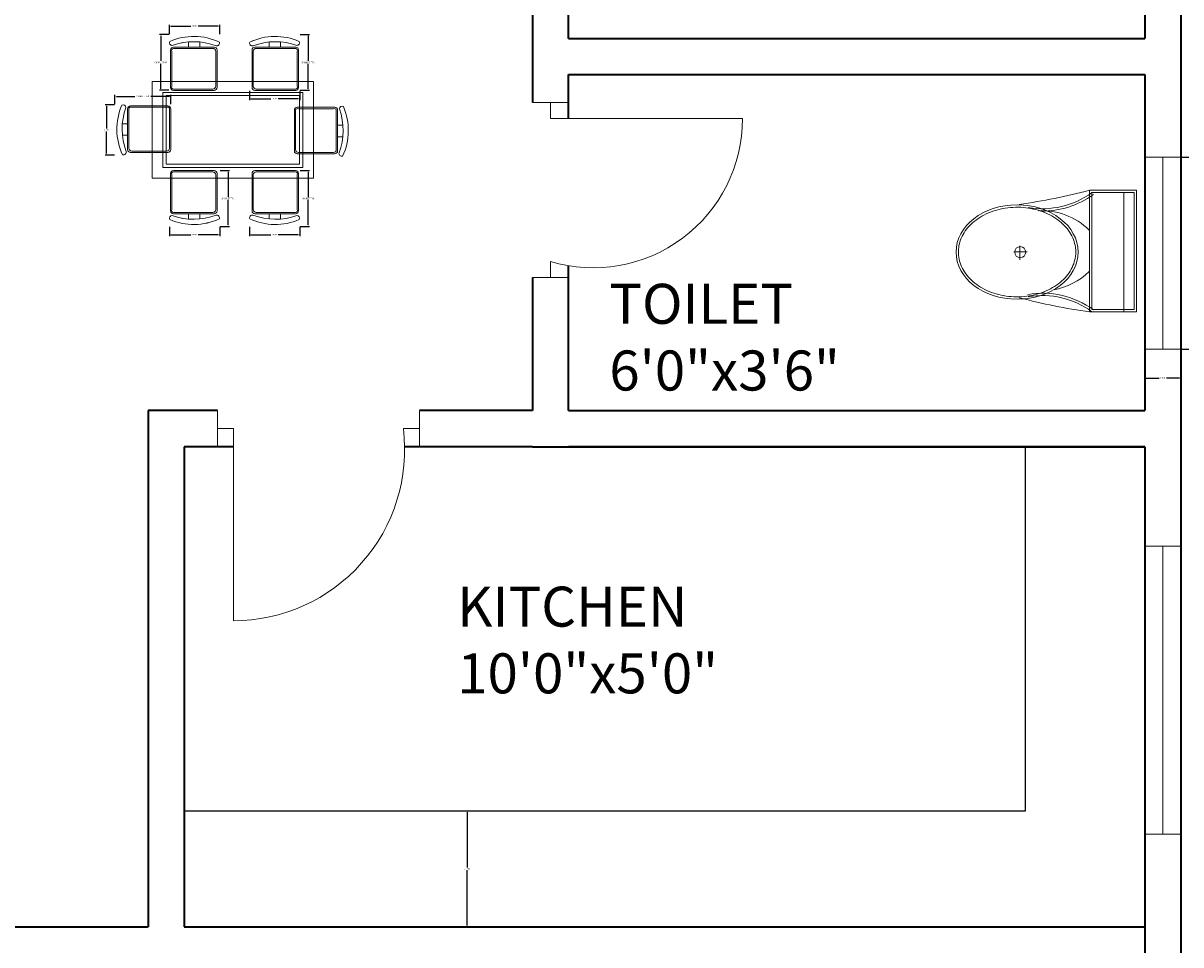
# Model space of a CAD drawing. Units: inches. Extents: x 2234 to 3001, y 1541 to 2386.
# Tile 10 of 12: x 2744 to 2888, y 2002 to 2118. Entities that reach past the tile are written whole.
import ezdxf

# ---------------------------------------------------------------- set-up
doc = ezdxf.new("R2010")
doc.units = ezdxf.units.IN
for name, color, linetype, lineweight in [('A-ANNO-DIMS', 2, 'Continuous', 18), ('A-AREA-IDEN', 7, 'Continuous', 18), ('A-DOOR', 3, 'Continuous', 18), ('A-FLOR-CASE', 8, 'Continuous', 25), ('A-FLOR-FIXT', 9, 'Continuous', 18), ('A-FURN', 9, 'Continuous', 13), ('A-GLAZ', 4, 'Continuous', 18), ('A-WALL', 7, 'Continuous', 35)]:
    doc.layers.add(name, color=color, linetype=linetype, lineweight=lineweight)
doc.styles.get("Standard").update_dxf_attribs({"font": 'arial.ttf'})
doc.dimstyles.get("Standard").update_dxf_attribs({"dimtxt": 0.18, "dimasz": 0.18, "dimexe": 0.18, "dimexo": 0.0625, "dimgap": 0.09, "dimtad": 0, "dimtih": 1, "dimtoh": 1, "dimdec": 4, "dimzin": 0, "dimdsep": 46, "dimtxsty": 'Standard', "dimcen": 0.09, "dimadec": 0, "dimazin": 0, "dimtfac": 1, "dimtdec": 4, "dimtofl": 0, "dimtmove": 0, "dimatfit": 3, "dimfxl": 1, "dimtolj": 1, "dimtzin": 0, "dimarcsym": 0})

# ---------------------------------------------------------------- blocks, each defined once
blk = doc.blocks.new('A$C31115884')
for p, q in [((283.1, 497.7), (223.4, 497.7)), ((257.5, 466.4), (257.5, 523.2)), ((0, 200), (0, 0)), ((520, 200), (0, 200)), ((520, 0), (520, 200)), ((10, 190), (10, 10)), ((510, 190), (10, 190)), ((510, 10), (510, 190)), ((510, 54.5), (0, 54.5)), ((10, 10), (510, 10)), ((0, 0), (520, 0))]:
    blk.add_line(p, q)
blk.add_circle((255.6, 496.4), 23.6)
for centre, radius, start, end in [((2777.7, -204.6), 2807, 165.4549, 171.7133), ((3237, 905), 2807, 188.2867, 194.5451), ((-294.5, 403.3), 364.7, 324.2091, 9.3499), ((-294.5, 403.3), 374.7, 324.2091, 9.3499), ((805.8, 403.3), 364.7, 170.6501, 215.7909), ((139.5, 406.2), 293.5, 315.8436, 2.6563), ((805.8, 403.3), 374.7, 179.2036, 215.7909), ((383.6, 406.2), 293.5, 190.2774, 224.1564)]:
    blk.add_arc(centre, radius, start, end)
blk.add_ellipse((256.2, 509.9), major_axis=(0, -260.7), ratio=0.772727)
blk.add_open_spline([(256.2, 259.2), (263.1, 259.2), (270, 259.7), (287.8, 262.3), (298.7, 265.1), (319.9, 273.1), (330.2, 278.4), (350.1, 291.1), (359.7, 298.7), (377.7, 315.9), (386.2, 325.5), (401.7, 346.6), (408.8, 358.1), (421.3, 382.5), (426.8, 395.5), (435.9, 422.4), (439.5, 436.4), (444.8, 465.1), (446.5, 479.7), (447.9, 509.2), (447.6, 524), (445, 553.3), (442.7, 567.8), (436.3, 596), (432.1, 609.7), (421.9, 636), (416, 648.6), (402.5, 672.1), (395, 683), (378.6, 703), (369.8, 712.1), (351.1, 728), (341.3, 734.8), (320.9, 746.2), (310.4, 750.7), (288.9, 757.3), (278, 759.4), (256, 761), (245, 760.6), (223.1, 757.2), (212.3, 754.3), (191.1, 746.1), (180.8, 740.7), (160.9, 727.8), (151.4, 720.1), (133.5, 702.7), (125.1, 693), (109.6, 671.7), (102.6, 660.2), (90.2, 635.7), (84.9, 622.7), (76, 595.6), (72.4, 581.6), (67.2, 552.9), (65.6, 538.2), (64.4, 508.8), (64.8, 494), (67.5, 464.7), (69.9, 450.2), (76.6, 422), (80.8, 408.3), (91.1, 382.2), (97.2, 369.7), (110.8, 346.3), (118.4, 335.4), (134.8, 315.6), (143.7, 306.7), (162.4, 290.9), (172.3, 284.2), (192.8, 273), (203.3, 268.6), (224.8, 262.2), (235.8, 260.2), (249.9, 259.3), (253, 259.2), (256.2, 259.2)], degree=3, knots=[0, 0, 0, 0, 0.110105, 0.110105, 0.285049, 0.285049, 0.459994, 0.459994, 0.634938, 0.634938, 0.809882, 0.809882, 0.984827, 0.984827, 1.159771, 1.159771, 1.334715, 1.334715, 1.50966, 1.50966, 1.684604, 1.684604, 1.859549, 1.859549, 2.034493, 2.034493, 2.209437, 2.209437, 2.384382, 2.384382, 2.559326, 2.559326, 2.73427, 2.73427, 2.909215, 2.909215, 3.084159, 3.084159, 3.259103, 3.259103, 3.434048, 3.434048, 3.608992, 3.608992, 3.783936, 3.783936, 3.958881, 3.958881, 4.133825, 4.133825, 4.30877, 4.30877, 4.483714, 4.483714, 4.658658, 4.658658, 4.833603, 4.833603, 5.008547, 5.008547, 5.183491, 5.183491, 5.358436, 5.358436, 5.53338, 5.53338, 5.708324, 5.708324, 5.883269, 5.883269, 6.058213, 6.058213, 6.233158, 6.233158, 6.283185, 6.283185, 6.283185, 6.283185])
blk = doc.blocks.new('TABLE-DINING-RECT')
for points in [[(0, 12.09), (20.14, 12.09), (20.14, 0), (0, 0)], [(0, 12.09), (20.14, 12.09), (20.14, 0), (0, 0)], [(1.34, 10.74), (18.8, 10.74), (18.8, 1.34), (1.34, 1.34)], [(1.34, 10.74), (18.8, 10.74), (18.8, 1.34), (1.34, 1.34)], [(1.75, 10.34), (18.4, 10.34), (18.4, 1.75), (1.75, 1.75)], [(1.75, 10.34), (18.4, 10.34), (18.4, 1.75), (1.75, 1.75)]]:
    blk.add_lwpolyline(points, close=True)
blk = doc.blocks.new('CHAIR-DINING-A')
for points in [[(5.76, 1.34, 0.414214), (6.12, 1.7), (6.12, 6.38, 0.414214), (5.76, 6.74), (0.67, 6.74, 0.414214), (0.31, 6.38), (0.31, 1.7, 0.414214), (0.67, 1.34), (5.76, 1.34)], [(5.76, 1.34, 0.414214), (6.12, 1.7), (6.12, 6.38, 0.414214), (5.76, 6.74), (0.67, 6.74, 0.414214), (0.31, 6.38), (0.31, 1.7, 0.414214), (0.67, 1.34), (5.76, 1.34)], [(5.92, 1.12, -0.175809), (0.43, 1.16, 0.578392), (0.02, 0.71, 0.214524), (6.21, 0.62, 0.552014), (5.92, 1.12, -0.065079)], [(5.92, 1.12, -0.175809), (0.43, 1.16, 0.578392), (0.02, 0.71, 0.214524), (6.21, 0.62, 0.552014), (5.92, 1.12, -0.065079)], [(2.45, 1.34), (2.45, 0.7, -0.064759)], [(2.45, 1.34), (2.45, 0.7, -0.064759)]]:
    blk.add_lwpolyline(points, format="xyb")
blk.add_lwpolyline([(5.76, 1.5), (0.83, 1.5, -0.414214), (0.47, 1.86), (0.47, 6.22, -0.414214), (0.83, 6.58), (5.76, 6.58, -0.512069), (5.95, 6.22), (5.95, 1.86, -0.512069)], format="xyb", close=True)
blk.add_lwpolyline([(5.76, 1.5), (0.83, 1.5, -0.414214), (0.47, 1.86), (0.47, 6.22, -0.414214), (0.83, 6.58), (5.76, 6.58, -0.512069), (5.95, 6.22), (5.95, 1.86, -0.512069)], format="xyb", close=True)
blk.add_lwpolyline([(3.88, 0.69), (3.88, 1.34)])
blk.add_lwpolyline([(3.88, 0.69), (3.88, 1.34)])
blk = doc.blocks.new('CHAIR-DINING-C')
for points in [[(1.16, 0.43, -0.578392), (0.71, 0.02, -0.214524), (0.62, 6.21, -0.552014), (1.12, 5.92, 0.175809), (1.16, 0.43)], [(1.34, 5.76, -0.414214), (1.7, 6.11), (6.38, 6.11, -0.414214), (6.74, 5.76), (6.74, 0.66, -0.414214), (6.38, 0.31), (1.7, 0.31, -0.414214), (1.34, 0.66), (1.34, 5.76)], [(1.34, 2.45), (0.7, 2.45, 0.064759)]]:
    blk.add_lwpolyline(points, format="xyb")
blk.add_lwpolyline([(1.5, 5.76), (1.5, 0.83, 0.414214), (1.86, 0.47), (6.22, 0.47, 0.414214), (6.58, 0.83), (6.58, 5.76, 0.512069), (6.22, 5.95), (1.86, 5.95, 0.512069)], format="xyb", close=True)
blk.add_lwpolyline([(0.69, 3.88), (1.34, 3.88)])
blk = doc.blocks.new('CHAIR-DINING-D')
for points in [[(0.43, 5.57, -0.578392), (0.02, 6.03, -0.214524), (6.21, 6.11, -0.552014), (5.92, 5.62, 0.175809), (0.43, 5.57)], [(2.45, 5.4), (2.45, 6.04, 0.064759)], [(5.76, 5.4, -0.414214), (6.12, 5.04), (6.12, 0.36, -0.414214), (5.76, 0), (0.67, 0, -0.414214), (0.31, 0.36), (0.31, 5.04, -0.414214), (0.67, 5.4), (5.76, 5.4)]]:
    blk.add_lwpolyline(points, format="xyb")
blk.add_lwpolyline([(3.88, 6.05), (3.88, 5.4)])
blk.add_lwpolyline([(5.76, 5.24), (0.83, 5.24, 0.414214), (0.47, 4.88), (0.47, 0.52, 0.414214), (0.83, 0.16), (5.76, 0.16, 0.512069), (5.95, 0.52), (5.95, 4.88, 0.512069)], format="xyb", close=True)
blk = doc.blocks.new('CHAIR-DINING-E')
for points in [[(5.76, 1.34, 0.414214), (6.12, 1.7), (6.12, 6.38, 0.414214), (5.76, 6.74), (0.67, 6.74, 0.414214), (0.31, 6.38), (0.31, 1.7, 0.414214), (0.67, 1.34), (5.76, 1.34)], [(5.92, 1.12, -0.175809), (0.43, 1.16, 0.578392), (0.02, 0.71, 0.214524), (6.21, 0.62, 0.552014), (5.92, 1.12, -0.065079)], [(2.45, 1.34), (2.45, 0.7, -0.064759)]]:
    blk.add_lwpolyline(points, format="xyb")
blk.add_lwpolyline([(5.76, 1.5), (0.83, 1.5, -0.414214), (0.47, 1.86), (0.47, 6.22, -0.414214), (0.83, 6.58), (5.76, 6.58, -0.512069), (5.95, 6.22), (5.95, 1.86, -0.512069)], format="xyb", close=True)
blk.add_lwpolyline([(3.88, 0.69), (3.88, 1.34)])
blk = doc.blocks.new('CHAIR-DINING-G')
for points in [[(5.58, 1.34), (0.49, 1.34, -0.414214), (0.13, 1.7), (0.13, 6.38, -0.414214), (0.49, 6.74), (5.58, 6.74, -0.414214), (5.94, 6.38), (5.94, 1.7, -0.414214), (5.58, 1.34)], [(5.82, 1.16, -0.578392), (6.23, 0.71, -0.214524), (0.04, 0.62, -0.552014), (0.33, 1.12, 0.175809), (5.82, 1.16)], [(3.79, 1.34), (3.79, 0.7, 0.064759)]]:
    blk.add_lwpolyline(points, format="xyb")
blk.add_lwpolyline([(0.49, 1.5), (5.42, 1.5, 0.414214), (5.78, 1.86), (5.78, 6.22, 0.414214), (5.42, 6.58), (0.49, 6.58, 0.512069), (0.29, 6.22), (0.29, 1.86, 0.512069)], format="xyb", close=True)
blk.add_lwpolyline([(2.37, 0.69), (2.37, 1.34)])
blk = doc.blocks.new('CHAIR-DINING-H')
for points in [[(1.16, 0.43, -0.578392), (0.71, 0.02, -0.214524), (0.62, 6.21, -0.552014), (1.12, 5.92, 0.175809), (1.16, 0.43)], [(1.34, 5.76, -0.414214), (1.7, 6.11), (6.38, 6.11, -0.414214), (6.74, 5.76), (6.74, 0.66, -0.414214), (6.38, 0.31), (1.7, 0.31, -0.414214), (1.34, 0.66), (1.34, 5.76)], [(1.34, 2.45), (0.7, 2.45, 0.064759)]]:
    blk.add_lwpolyline(points, format="xyb")
blk.add_lwpolyline([(1.5, 5.76), (1.5, 0.83, 0.414214), (1.86, 0.47), (6.22, 0.47, 0.414214), (6.58, 0.83), (6.58, 5.76, 0.512069), (6.22, 5.95), (1.86, 5.95, 0.512069)], format="xyb", close=True)
blk.add_lwpolyline([(0.69, 3.88), (1.34, 3.88)])
blk = doc.blocks.new('CHAIR-DINING-I')
for points in [[(0.33, 5.62, -0.175809), (5.82, 5.57, 0.578392), (6.23, 6.03, 0.214524), (0.04, 6.11, 0.552014), (0.33, 5.62, -0.065079)], [(3.79, 5.4), (3.79, 6.04, -0.064759)], [(5.58, 5.4), (0.49, 5.4, 0.414214), (0.13, 5.04), (0.13, 0.36, 0.414214), (0.49, 0), (5.58, 0, 0.414214), (5.94, 0.36), (5.94, 5.04, 0.414214), (5.58, 5.4)]]:
    blk.add_lwpolyline(points, format="xyb")
blk.add_lwpolyline([(2.37, 6.05), (2.37, 5.4)])
blk.add_lwpolyline([(0.49, 5.24), (5.42, 5.24, -0.414214), (5.78, 4.88), (5.78, 0.52, -0.414214), (5.42, 0.16), (0.49, 0.16, -0.512069), (0.29, 0.52), (0.29, 4.88, -0.512069)], format="xyb", close=True)
blk = doc.blocks.new('WIN-24-A')
for p, q in [((0, 24), (4.5, 24)), ((4.5, 24), (2.25, 24)), ((2.25, 24), (2.25, 0)), ((2.25, 0), (0, 0)), ((0, 0), (4.5, 0))]:
    blk.add_line(p, q)
blk = doc.blocks.new('WIN-36')
for p, q in [((0, 36), (4.5, 36)), ((4.5, 36), (2.25, 36)), ((2.25, 36), (2.25, 0)), ((2.25, 0), (0, 0)), ((0, 0), (4.5, 0))]:
    blk.add_line(p, q)
blk = doc.blocks.new('*D29')
at = {"layer": 'A-ANNO-DIMS', "color": 0, "lineweight": -2, "transparency": 16777216}
for p, q in [((2888.32, 2100.78), (2892.03, 2100.78)), ((2891.85, 2100.6), (2891.85, 2088.96)), ((2891.85, 2076.96), (2891.85, 2088.6)), ((2888.32, 2076.78), (2892.03, 2076.78))]:
    blk.add_line(p, q, dxfattribs=at)
at = {"layer": 'A-ANNO-DIMS', "color": 0, "transparency": 16777216}
for points in [[(2891.82, 2100.6), (2891.88, 2100.6), (2891.85, 2100.78)], [(2891.82, 2076.96), (2891.88, 2076.96), (2891.85, 2076.78)]]:
    blk.add_solid(points, dxfattribs=at)
at = {"layer": 'Defpoints', "color": 0, "transparency": 16777216}
for p in [(2888.25, 2100.78), (2888.25, 2076.78), (2891.85, 2076.78)]:
    blk.add_point(p, dxfattribs=at)
at = {"layer": 'A-ANNO-DIMS', "color": 0, "transparency": 16777216, "insert": (2891.85, 2088.78), "char_height": 0.18, "attachment_point": 5}
blk.add_mtext('\\A1;W-A 24 TYP.', dxfattribs=at)
blk = doc.blocks.new('*D30')
at = {"layer": 'A-ANNO-DIMS', "color": 0, "lineweight": -2, "transparency": 16777216}
for p, q in [((2883.75, 2076.72), (2883.75, 2073)), ((2888.25, 2076.72), (2888.25, 2073)), ((2883.93, 2073.18), (2885.55, 2073.18)), ((2888.07, 2073.18), (2886.46, 2073.18))]:
    blk.add_line(p, q, dxfattribs=at)
at = {"layer": 'A-ANNO-DIMS', "color": 0, "transparency": 16777216}
for points in [[(2883.93, 2073.21), (2883.93, 2073.15), (2883.75, 2073.18)], [(2888.07, 2073.21), (2888.07, 2073.15), (2888.25, 2073.18)]]:
    blk.add_solid(points, dxfattribs=at)
at = {"layer": 'Defpoints', "color": 0, "transparency": 16777216}
for p in [(2883.75, 2076.78), (2888.25, 2076.78), (2883.75, 2073.18)]:
    blk.add_point(p, dxfattribs=at)
at = {"layer": 'A-ANNO-DIMS', "color": 0, "transparency": 16777216, "insert": (2886, 2073.18), "char_height": 0.18, "attachment_point": 5}
blk.add_mtext('\\A1;5 TYP.', dxfattribs=at)
blk = doc.blocks.new('*D47')
at = {"layer": 'A-ANNO-DIMS', "color": 0, "lineweight": -2, "transparency": 16777216}
for p, q in [((2778.25, 2116.11), (2779.41, 2116.11)), ((2779.23, 2115.93), (2779.23, 2112.81)), ((2779.23, 2109.32), (2779.23, 2112.44)), ((2778.25, 2109.14), (2779.41, 2109.14))]:
    blk.add_line(p, q, dxfattribs=at)
at = {"layer": 'A-ANNO-DIMS', "color": 0, "transparency": 16777216}
for points in [[(2779.2, 2115.93), (2779.26, 2115.93), (2779.23, 2116.11)], [(2779.2, 2109.32), (2779.26, 2109.32), (2779.23, 2109.14)]]:
    blk.add_solid(points, dxfattribs=at)
at = {"layer": 'Defpoints', "color": 0, "transparency": 16777216}
for p in [(2778.18, 2116.11), (2779.23, 2116.11), (2778.18, 2109.14)]:
    blk.add_point(p, dxfattribs=at)
at = {"layer": 'A-ANNO-DIMS', "color": 0, "transparency": 16777216, "insert": (2779.23, 2112.62), "char_height": 0.18, "attachment_point": 5}
blk.add_mtext('\\A1;CHAIR D 7 TYP.', dxfattribs=at)
blk = doc.blocks.new('*D48')
at = {"layer": 'A-ANNO-DIMS', "color": 0, "lineweight": -2, "transparency": 16777216}
for p, q in [((2771.9, 2109.07), (2771.9, 2107.91)), ((2778.18, 2109.07), (2778.18, 2107.91)), ((2772.08, 2108.09), (2774.58, 2108.09)), ((2778, 2108.09), (2775.5, 2108.09))]:
    blk.add_line(p, q, dxfattribs=at)
at = {"layer": 'A-ANNO-DIMS', "color": 0, "transparency": 16777216}
for points in [[(2772.08, 2108.12), (2772.08, 2108.06), (2771.9, 2108.09)], [(2778, 2108.12), (2778, 2108.06), (2778.18, 2108.09)]]:
    blk.add_solid(points, dxfattribs=at)
at = {"layer": 'Defpoints', "color": 0, "transparency": 16777216}
for p in [(2771.9, 2109.14), (2778.18, 2109.14), (2778.18, 2108.09)]:
    blk.add_point(p, dxfattribs=at)
at = {"layer": 'A-ANNO-DIMS', "color": 0, "transparency": 16777216, "insert": (2775.04, 2108.09), "char_height": 0.18, "attachment_point": 5}
blk.add_mtext('\\A1;6 TYP.', dxfattribs=at)
blk = doc.blocks.new('*D49')
at = {"layer": 'A-ANNO-DIMS', "color": 0, "lineweight": -2, "transparency": 16777216}
for p, q in [((2778.25, 2099.11), (2779.41, 2099.11)), ((2779.23, 2098.93), (2779.23, 2095.8)), ((2779.23, 2092.31), (2779.23, 2095.44)), ((2778.25, 2092.13), (2779.41, 2092.13))]:
    blk.add_line(p, q, dxfattribs=at)
at = {"layer": 'A-ANNO-DIMS', "color": 0, "transparency": 16777216}
for points in [[(2779.2, 2098.93), (2779.26, 2098.93), (2779.23, 2099.11)], [(2779.2, 2092.31), (2779.26, 2092.31), (2779.23, 2092.13)]]:
    blk.add_solid(points, dxfattribs=at)
at = {"layer": 'Defpoints', "color": 0, "transparency": 16777216}
for p in [(2778.18, 2099.11), (2779.23, 2099.11), (2778.18, 2092.13)]:
    blk.add_point(p, dxfattribs=at)
at = {"layer": 'A-ANNO-DIMS', "color": 0, "transparency": 16777216, "insert": (2779.23, 2095.62), "char_height": 0.18, "attachment_point": 5}
blk.add_mtext('\\A1;CHAIR E 7 TYP.', dxfattribs=at)
blk = doc.blocks.new('*D50')
at = {"layer": 'A-ANNO-DIMS', "color": 0, "lineweight": -2, "transparency": 16777216}
for p, q in [((2771.9, 2092.07), (2771.9, 2090.91)), ((2778.18, 2092.07), (2778.18, 2090.91)), ((2772.08, 2091.09), (2774.58, 2091.09)), ((2778, 2091.09), (2775.5, 2091.09))]:
    blk.add_line(p, q, dxfattribs=at)
at = {"layer": 'A-ANNO-DIMS', "color": 0, "transparency": 16777216}
for points in [[(2772.08, 2091.12), (2772.08, 2091.06), (2771.9, 2091.09)], [(2778, 2091.12), (2778, 2091.06), (2778.18, 2091.09)]]:
    blk.add_solid(points, dxfattribs=at)
at = {"layer": 'Defpoints', "color": 0, "transparency": 16777216}
for p in [(2771.9, 2092.13), (2778.18, 2092.13), (2778.18, 2091.09)]:
    blk.add_point(p, dxfattribs=at)
at = {"layer": 'A-ANNO-DIMS', "color": 0, "transparency": 16777216, "insert": (2775.04, 2091.09), "char_height": 0.18, "attachment_point": 5}
blk.add_mtext('\\A1;6 TYP.', dxfattribs=at)
blk = doc.blocks.new('*D53')
at = {"layer": 'A-ANNO-DIMS', "color": 0, "lineweight": -2, "transparency": 16777216}
for p, q in [((2768.25, 2099.11), (2769.41, 2099.11)), ((2769.23, 2098.93), (2769.23, 2095.8)), ((2769.23, 2092.31), (2769.23, 2095.44)), ((2768.25, 2092.13), (2769.41, 2092.13))]:
    blk.add_line(p, q, dxfattribs=at)
at = {"layer": 'A-ANNO-DIMS', "color": 0, "transparency": 16777216}
for points in [[(2769.2, 2098.93), (2769.26, 2098.93), (2769.23, 2099.11)], [(2769.2, 2092.31), (2769.26, 2092.31), (2769.23, 2092.13)]]:
    blk.add_solid(points, dxfattribs=at)
at = {"layer": 'Defpoints', "color": 0, "transparency": 16777216}
for p in [(2768.19, 2099.11), (2769.23, 2099.11), (2768.19, 2092.13)]:
    blk.add_point(p, dxfattribs=at)
at = {"layer": 'A-ANNO-DIMS', "color": 0, "transparency": 16777216, "insert": (2769.23, 2095.62), "char_height": 0.18, "attachment_point": 5}
blk.add_mtext('\\A1;CHAIR G 7 TYP.', dxfattribs=at)
blk = doc.blocks.new('*D54')
at = {"layer": 'A-ANNO-DIMS', "color": 0, "lineweight": -2, "transparency": 16777216}
for p, q in [((2761.9, 2092.07), (2761.9, 2090.91)), ((2768.19, 2092.07), (2768.19, 2090.91)), ((2762.08, 2091.09), (2764.59, 2091.09)), ((2768.01, 2091.09), (2765.5, 2091.09))]:
    blk.add_line(p, q, dxfattribs=at)
at = {"layer": 'A-ANNO-DIMS', "color": 0, "transparency": 16777216}
for points in [[(2762.08, 2091.12), (2762.08, 2091.06), (2761.9, 2091.09)], [(2768.01, 2091.12), (2768.01, 2091.06), (2768.19, 2091.09)]]:
    blk.add_solid(points, dxfattribs=at)
at = {"layer": 'Defpoints', "color": 0, "transparency": 16777216}
for p in [(2761.9, 2092.13), (2768.19, 2092.13), (2768.19, 2091.09)]:
    blk.add_point(p, dxfattribs=at)
at = {"layer": 'A-ANNO-DIMS', "color": 0, "transparency": 16777216, "insert": (2765.04, 2091.09), "char_height": 0.18, "attachment_point": 5}
blk.add_mtext('\\A1;6 TYP.', dxfattribs=at)
blk = doc.blocks.new('*D55')
at = {"layer": 'A-ANNO-DIMS', "color": 0, "lineweight": -2, "transparency": 16777216}
for p, q in [((2755.11, 2107.4), (2755.11, 2108.56)), ((2762.08, 2107.4), (2762.08, 2108.56)), ((2755.29, 2108.38), (2757.58, 2108.38)), ((2761.9, 2108.38), (2759.6, 2108.38))]:
    blk.add_line(p, q, dxfattribs=at)
at = {"layer": 'A-ANNO-DIMS', "color": 0, "transparency": 16777216}
for points in [[(2755.29, 2108.41), (2755.29, 2108.35), (2755.11, 2108.38)], [(2761.9, 2108.41), (2761.9, 2108.35), (2762.08, 2108.38)]]:
    blk.add_solid(points, dxfattribs=at)
at = {"layer": 'Defpoints', "color": 0, "transparency": 16777216}
for p in [(2755.11, 2107.33), (2762.08, 2108.38), (2762.08, 2107.33)]:
    blk.add_point(p, dxfattribs=at)
at = {"layer": 'A-ANNO-DIMS', "color": 0, "transparency": 16777216, "insert": (2758.59, 2108.38), "char_height": 0.18, "attachment_point": 5}
blk.add_mtext('\\A1;CHAIR H 7 TYP.', dxfattribs=at)
blk = doc.blocks.new('*D56')
at = {"layer": 'A-ANNO-DIMS', "color": 0, "lineweight": -2, "transparency": 16777216}
for p, q in [((2755.04, 2107.33), (2753.88, 2107.33)), ((2754.06, 2107.15), (2754.06, 2104.37)), ((2754.06, 2101.23), (2754.06, 2104.01)), ((2755.04, 2101.05), (2753.88, 2101.05))]:
    blk.add_line(p, q, dxfattribs=at)
at = {"layer": 'A-ANNO-DIMS', "color": 0, "transparency": 16777216}
for points in [[(2754.03, 2107.15), (2754.09, 2107.15), (2754.06, 2107.33)], [(2754.03, 2101.23), (2754.09, 2101.23), (2754.06, 2101.05)]]:
    blk.add_solid(points, dxfattribs=at)
at = {"layer": 'Defpoints', "color": 0, "transparency": 16777216}
for p in [(2754.06, 2107.33), (2755.11, 2107.33), (2755.11, 2101.05)]:
    blk.add_point(p, dxfattribs=at)
at = {"layer": 'A-ANNO-DIMS', "color": 0, "transparency": 16777216, "insert": (2754.06, 2104.19), "char_height": 0.18, "attachment_point": 5}
blk.add_mtext('\\A1;6 TYP.', dxfattribs=at)
blk = doc.blocks.new('*D57')
at = {"layer": 'A-ANNO-DIMS', "color": 0, "lineweight": -2, "transparency": 16777216}
for p, q in [((2761.84, 2116.11), (2760.67, 2116.11)), ((2760.85, 2115.93), (2760.85, 2112.81)), ((2760.85, 2109.32), (2760.85, 2112.44)), ((2761.84, 2109.14), (2760.67, 2109.14))]:
    blk.add_line(p, q, dxfattribs=at)
at = {"layer": 'A-ANNO-DIMS', "color": 0, "transparency": 16777216}
for points in [[(2760.82, 2115.93), (2760.88, 2115.93), (2760.85, 2116.11)], [(2760.82, 2109.32), (2760.88, 2109.32), (2760.85, 2109.14)]]:
    blk.add_solid(points, dxfattribs=at)
at = {"layer": 'Defpoints', "color": 0, "transparency": 16777216}
for p in [(2760.85, 2116.11), (2761.9, 2116.11), (2761.9, 2109.14)]:
    blk.add_point(p, dxfattribs=at)
at = {"layer": 'A-ANNO-DIMS', "color": 0, "transparency": 16777216, "insert": (2760.85, 2112.62), "char_height": 0.18, "attachment_point": 5}
blk.add_mtext('\\A1;CHAIR I 7 TYP.', dxfattribs=at)
blk = doc.blocks.new('*D58')
at = {"layer": 'A-ANNO-DIMS', "color": 0, "lineweight": -2, "transparency": 16777216}
for p, q in [((2761.9, 2116.17), (2761.9, 2117.34)), ((2768.19, 2116.17), (2768.19, 2117.34)), ((2762.08, 2117.16), (2764.59, 2117.16)), ((2768.01, 2117.16), (2765.5, 2117.16))]:
    blk.add_line(p, q, dxfattribs=at)
at = {"layer": 'A-ANNO-DIMS', "color": 0, "transparency": 16777216}
for points in [[(2762.08, 2117.19), (2762.08, 2117.13), (2761.9, 2117.16)], [(2768.01, 2117.19), (2768.01, 2117.13), (2768.19, 2117.16)]]:
    blk.add_solid(points, dxfattribs=at)
at = {"layer": 'Defpoints', "color": 0, "transparency": 16777216}
for p in [(2761.9, 2116.11), (2768.19, 2117.16), (2768.19, 2116.11)]:
    blk.add_point(p, dxfattribs=at)
at = {"layer": 'A-ANNO-DIMS', "color": 0, "transparency": 16777216, "insert": (2765.04, 2117.16), "char_height": 0.18, "attachment_point": 5}
blk.add_mtext('\\A1;6 TYP.', dxfattribs=at)
blk = doc.blocks.new('*D73')
at = {"layer": 'A-ANNO-DIMS', "color": 0, "lineweight": -2, "transparency": 16777216}
for p, q in [((2763.82, 2019.11), (2799.28, 2019.11)), ((2799.1, 2018.93), (2799.1, 2012.04)), ((2799.1, 2004.79), (2799.1, 2011.68)), ((2763.82, 2004.61), (2799.28, 2004.61))]:
    blk.add_line(p, q, dxfattribs=at)
at = {"layer": 'A-ANNO-DIMS', "color": 0, "transparency": 16777216}
for points in [[(2799.07, 2018.93), (2799.13, 2018.93), (2799.1, 2019.11)], [(2799.07, 2004.79), (2799.13, 2004.79), (2799.1, 2004.61)]]:
    blk.add_solid(points, dxfattribs=at)
at = {"layer": 'Defpoints', "color": 0, "transparency": 16777216}
for p in [(2763.75, 2019.11), (2763.75, 2004.61), (2799.1, 2004.61)]:
    blk.add_point(p, dxfattribs=at)
at = {"layer": 'A-ANNO-DIMS', "color": 0, "transparency": 16777216, "insert": (2799.1, 2011.86), "char_height": 0.18, "attachment_point": 5}
blk.add_mtext('\\A1;14.498', dxfattribs=at)

msp = doc.modelspace()

# ---------------------------------------------------------------- linework, layer by layer
at = {"layer": 'A-DOOR'}
for p, q in [((2811.7534, 2107.6086), (2807.2534, 2107.6086)), ((2807.2534, 2107.6086), (2809.5034, 2107.6086)), ((2809.5034, 2107.6086), (2809.5034, 2105.6086)), ((2809.5034, 2105.6086), (2833.5034, 2105.6086)), ((2809.5034, 2085.7488), (2809.5034, 2087.7488)), ((2811.7534, 2085.7488), (2807.2534, 2085.7488)), ((2807.2534, 2085.7488), (2809.5034, 2085.7488)), ((2767.8978, 2064.611), (2767.8978, 2069.111)), ((2767.8978, 2069.111), (2767.8978, 2066.861)), ((2793.1311, 2064.611), (2793.1311, 2069.111)), ((2793.1311, 2069.111), (2793.1311, 2066.861)), ((2767.8978, 2066.861), (2769.8978, 2066.861)), ((2769.8978, 2066.861), (2769.8978, 2042.861)), ((2793.1311, 2066.861), (2791.1311, 2066.861))]:
    msp.add_line(p, q, dxfattribs=at)
for centre, radius, start, end in [((2814.8582, 2105.6086), 18.6453, 253.310145, 0), ((2769.8978, 2064.2539), 21.3928, 270, 7.000088)]:
    msp.add_arc(centre, radius, start, end, dxfattribs=at)
at = {"layer": 'A-FLOR-CASE'}
for p, q in [((2868.8394, 2019.1088), (2868.8394, 2064.611)), ((2763.7534, 2019.1088), (2868.8394, 2019.1088))]:
    msp.add_line(p, q, dxfattribs=at)
at = {"layer": 'A-FURN'}
for points in [[(2762.2461, 2114.7519, -0.17580919), (2767.7328, 2114.7104, 0.57839206), (2768.1484, 2115.1674, 0.21452438), (2761.9552, 2115.2505, 0.55201397), (2762.2461, 2114.7519, -0.06507904)], [(2772.3518, 2114.7104, -0.57839206), (2771.9361, 2115.1674, -0.21452438), (2778.1294, 2115.2505, -0.55201397), (2777.8384, 2114.7519, 0.1758092), (2772.3518, 2114.7104)], [(2767.5, 2114.5317), (2762.4064, 2114.5317, 0.41421356), (2762.05, 2114.1754), (2762.05, 2109.4919, 0.41421356), (2762.4064, 2109.1355), (2767.5, 2109.1355, 0.41421356), (2767.8563, 2109.4919), (2767.8563, 2114.1754, 0.41421356), (2767.5, 2114.5317)], [(2765.7109, 2114.5317), (2765.7109, 2115.1759, -0.06475861)], [(2777.6782, 2114.5317, -0.41421356), (2778.0345, 2114.1754), (2778.0345, 2109.4919, -0.41421356), (2777.6782, 2109.1355), (2772.5846, 2109.1355, -0.41421356), (2772.2282, 2109.4919), (2772.2282, 2114.1754, -0.41421356), (2772.5846, 2114.5317), (2777.6782, 2114.5317)], [(2774.3737, 2114.5317), (2774.3737, 2115.1759, 0.06475861)], [(2767.5, 2093.7125), (2762.4064, 2093.7125, -0.41421356), (2762.05, 2094.0689), (2762.05, 2098.7524, -0.41421356), (2762.4064, 2099.1087), (2767.5, 2099.1087, -0.41421356), (2767.8563, 2098.7524), (2767.8563, 2094.0689, -0.41421356), (2767.5, 2093.7125)], [(2767.7328, 2093.5339, -0.57839206), (2768.1484, 2093.0768, -0.21452438), (2761.9552, 2092.9937, -0.55201397), (2762.2461, 2093.4923, 0.17580929), (2767.7328, 2093.5339)], [(2765.7109, 2093.7125), (2765.7109, 2093.0683, 0.06475861)]]:
    msp.add_lwpolyline(points, format="xyb", dxfattribs=at)
for points in [[(2762.4085, 2114.3712), (2767.3394, 2114.3712, -0.41421356), (2767.6958, 2114.0148), (2767.6958, 2109.6524, -0.41421356), (2767.3394, 2109.2961), (2762.4085, 2109.2961, -0.51206948), (2762.2106, 2109.6524), (2762.2106, 2114.0148, -0.51206948)], [(2777.676, 2114.3712), (2772.7451, 2114.3712, 0.41421356), (2772.3888, 2114.0148), (2772.3888, 2109.6524, 0.41421356), (2772.7451, 2109.2961), (2777.676, 2109.2961, 0.51206948), (2777.874, 2109.6524), (2777.874, 2114.0148, 0.51206948)], [(2762.4085, 2093.8731), (2767.3394, 2093.8731, 0.41421356), (2767.6958, 2094.2294), (2767.6958, 2098.5918, 0.41421356), (2767.3394, 2098.9482), (2762.4085, 2098.9482, 0.51206948), (2762.2106, 2098.5918), (2762.2106, 2094.2294, 0.51206948)]]:
    msp.add_lwpolyline(points, format="xyb", close=True, dxfattribs=at)
for points in [[(2764.2851, 2115.1876), (2764.2851, 2114.5317)], [(2775.7995, 2115.1876), (2775.7995, 2114.5317)], [(2764.2851, 2093.0566), (2764.2851, 2093.7125)]]:
    msp.add_lwpolyline(points, dxfattribs=at)
at = {"layer": 'A-WALL'}
for p, q in [((2888.2534, 2298.611), (2888.2534, 1702.111)), ((2807.2534, 2157.611), (2807.2534, 2107.6086)), ((2811.7534, 2115.611), (2811.7534, 2157.611)), ((2883.7534, 2157.611), (2883.7534, 2115.611)), ((2811.7534, 2115.611), (2883.7534, 2115.611)), ((2811.7534, 2111.111), (2883.7534, 2111.111)), ((2811.7534, 2105.6086), (2811.7534, 2111.111)), ((2883.7534, 2111.111), (2883.7534, 2069.111)), ((2811.7534, 2069.111), (2811.7534, 2087.2236)), ((2807.2534, 2085.7488), (2807.2534, 2069.111)), ((2759.2534, 2069.111), (2759.2534, 2064.611)), ((2767.8978, 2069.111), (2759.2534, 2069.111)), ((2807.2534, 2069.111), (2793.1311, 2069.111)), ((2811.7534, 2069.111), (2883.7534, 2069.111)), ((2759.2534, 2064.611), (2759.2534, 2004.611)), ((2763.7534, 2064.611), (2763.7534, 2004.611)), ((2769.8978, 2064.611), (2763.7534, 2064.611)), ((2807.2534, 2064.611), (2791.2876, 2064.611)), ((2807.2534, 2064.611), (2883.7534, 2064.611)), ((2883.7534, 2064.611), (2811.7534, 2064.611)), ((2883.7534, 2064.611), (2883.7534, 1940.111)), ((2636.7879, 2004.611), (2759.2534, 2004.611)), ((2763.7534, 2004.611), (2883.7534, 2004.611))]:
    msp.add_line(p, q, dxfattribs=at)

# ---------------------------------------------------------------- block references
at = {"layer": 'A-FLOR-FIXT', "xscale": 0.0292470664339069, "yscale": 0.0292470664339069, "zscale": 0.0292470664339069, "rotation": 89.99999999999999}
msp.add_blockref('A$C31115884', (2882.7092, 2081.4404), dxfattribs=at)
at = {"layer": 'A-FURN'}
for name, p in [('CHAIR-DINING-I', (2761.9165, 2109.1359)), ('CHAIR-DINING-D', (2771.9195, 2109.1359)), ('TABLE-DINING-RECT', (2759.7543, 2098.1438)), ('CHAIR-DINING-H', (2755.3435, 2101.0707)), ('CHAIR-DINING-C', (2755.3434, 2101.0707)), ('CHAIR-DINING-G', (2761.9165, 2092.3717)), ('CHAIR-DINING-E', (2771.919, 2092.3712)), ('CHAIR-DINING-E', (2771.919, 2092.371))]:
    msp.add_blockref(name, p, dxfattribs=at)
at = {"layer": 'A-FURN', "rotation": 90}
msp.add_blockref('CHAIR-DINING-A', (2784.2563, 2100.8957), dxfattribs=at)
at = {"layer": 'A-GLAZ', "rotation": 180}
msp.add_blockref('WIN-24-A', (2888.2539, 2100.779), dxfattribs=at)
at = {"layer": 'A-GLAZ'}
msp.add_blockref('WIN-36', (2883.753, 2016.1757), dxfattribs=at)

# ---------------------------------------------------------------- texts
at = {"layer": 'A-AREA-IDEN', "char_height": 5, "attachment_point": 1}
for s, width, insert in [('TOILET\\P6\'0"x3\'6"', 103.95506, (2816.8625, 2084.9623)), ('KITCHEN\\P10\'0"x5\'0"', 106.174758, (2797.8638, 2047.1218))]:
    msp.add_mtext_dynamic_manual_height_columns(s, width=width, gutter_width=12.5, heights=[0], dxfattribs=dict(at, insert=insert))

# ---------------------------------------------------------------- dimensions: what is measured, and where the dimension line sits
at = {"layer": 'A-ANNO-DIMS'}
for base, p1, p2, text, picture, middle in [((2768.1874, 2117.1562), (2761.901, 2116.11), (2768.1874, 2116.11), '<> TYP.', '*D58', (2765.0442, 2117.1562)), ((2762.0809, 2108.3807), (2755.1066, 2107.3345), (2762.0809, 2107.3345), 'CHAIR H <> TYP.', '*D55', (2758.5937, 2108.3807)), ((2778.1836, 2108.0896), (2771.8971, 2109.1357), (2778.1836, 2109.1357), '<> TYP.', '*D48', (2775.0404, 2108.0896)), ((2768.1874, 2091.0885), (2761.901, 2092.1346), (2768.1874, 2092.1346), '<> TYP.', '*D54', (2765.0442, 2091.0885)), ((2778.1836, 2091.0883), (2771.8972, 2092.1344), (2778.1836, 2092.1344), '<> TYP.', '*D50', (2775.0404, 2091.0883))]:
    dim = msp.add_linear_dim(base=base, p1=p1, p2=p2, text=text, dimstyle='Standard', override={"dimdec": 0, "dimlfac": 1, "dimrnd": 0, "dimzin": 0, "dimdsep": 46, "dimlunit": 2}, dxfattribs=at)
    dim.commit()
    dim.dimension.update_dxf_attribs({"geometry": picture, "text_midpoint": middle})
for base, p1, p2, angle, text, picture, middle in [((2760.8548, 2116.11), (2761.901, 2109.1357), (2761.901, 2116.11), 90, 'CHAIR I <> TYP.', '*D57', (2760.8548, 2112.6229)), ((2779.2297, 2116.11), (2778.1836, 2109.1357), (2778.1836, 2116.11), 90, 'CHAIR D <> TYP.', '*D47', (2779.2297, 2112.6229)), ((2754.0604, 2107.3345), (2755.1066, 2101.0481), (2755.1066, 2107.3345), 90, '<> TYP.', '*D56', (2754.0604, 2104.1913)), ((2891.8534, 2076.7794), (2888.2534, 2100.7794), (2888.2534, 2076.7794), 270, 'W-A <> TYP.', '*D29', (2891.8534, 2088.7794)), ((2769.2335, 2099.1089), (2768.1874, 2092.1346), (2768.1874, 2099.1089), 90, 'CHAIR G <> TYP.', '*D53', (2769.2335, 2095.6218)), ((2779.2297, 2099.1087), (2778.1836, 2092.1344), (2778.1836, 2099.1087), 90, 'CHAIR E <> TYP.', '*D49', (2779.2297, 2095.6216)), ((2883.7534479173, 2073.1793646181), (2888.2534479174, 2076.7793646181), (2883.7534479173, 2076.7793646181), 180, '<> TYP.', '*D30', (2886.0034479173, 2073.1793646181))]:
    dim = msp.add_linear_dim(base=base, p1=p1, p2=p2, angle=angle, text=text, dimstyle='Standard', override={"dimdec": 0, "dimlfac": 1, "dimrnd": 0, "dimzin": 0, "dimdsep": 46, "dimlunit": 2}, dxfattribs=at)
    dim.commit()
    dim.dimension.update_dxf_attribs({"geometry": picture, "text_midpoint": middle})
dim = msp.add_linear_dim(base=(2799.1034, 2004.611), p1=(2763.7534, 2019.1088), p2=(2763.7534, 2004.611), angle=270, dimstyle='Standard', override={"dimdec": 3, "dimlfac": 1, "dimrnd": 0, "dimzin": 0, "dimdsep": 46, "dimlunit": 2}, dxfattribs=at)
dim.commit()
dim.dimension.update_dxf_attribs({"geometry": '*D73', "text_midpoint": (2799.1034, 2011.8599)})

doc.saveas('drawing.dxf')
